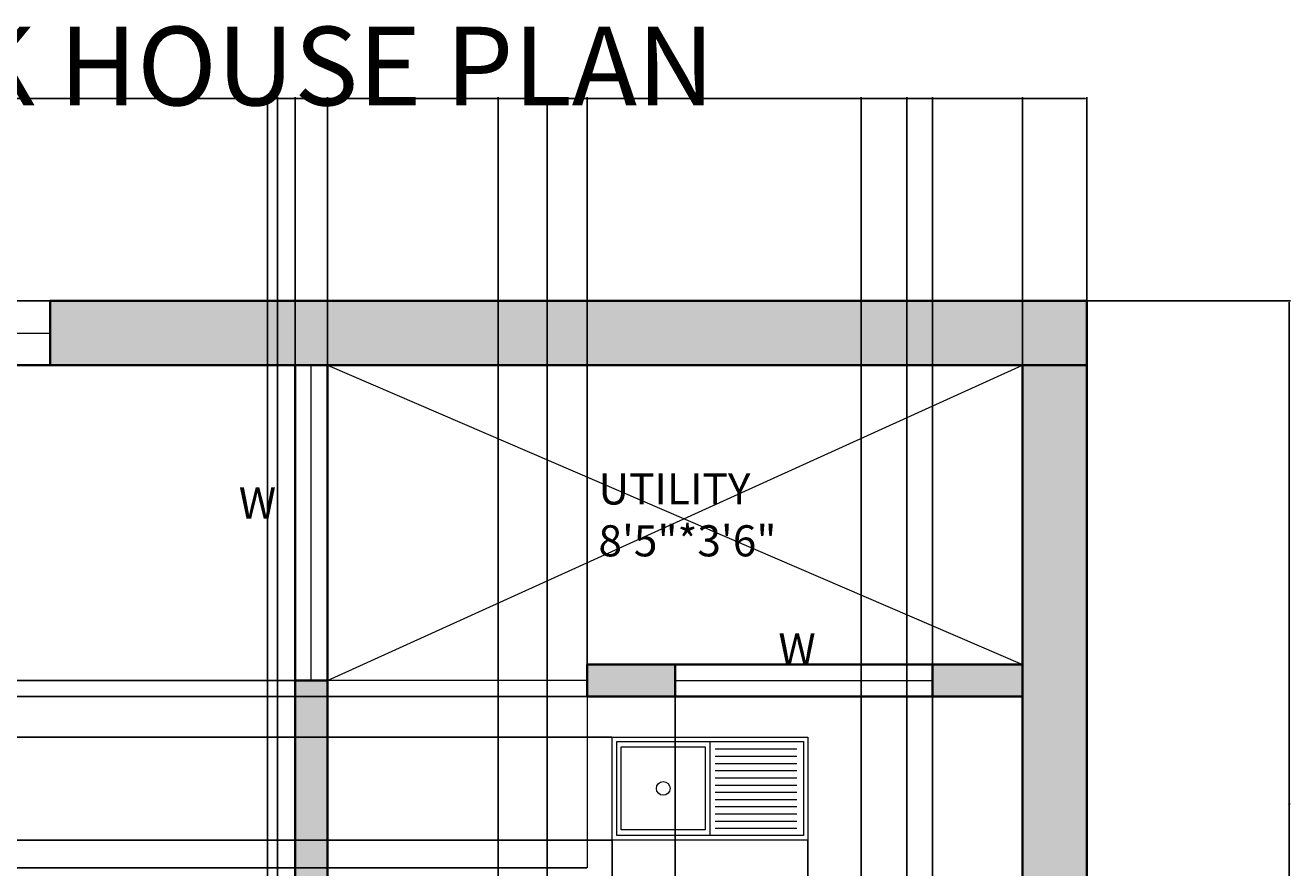
# Model space of a CAD drawing. Units: inches. Extents: x 2035 to 2384, y 1427 to 2020.
# Tile 7 of 7: x 2206 to 2383, y 1902 to 2020. Entities that reach past the tile are written whole.
import ezdxf

# ---------------------------------------------------------------- set-up
doc = ezdxf.new("R2010")
doc.units = ezdxf.units.IN
for name, color, linetype, lineweight in [('A-ANNO-DIMS', 2, 'Continuous', 18), ('A-ANNO-IDEN', 201, 'Continuous', 18), ('A-ANNO-TITL', 7, 'Continuous', 35), ('A-AREA-IDEN', 201, 'Continuous', 18), ('A-FLOR-CABN', 71, 'Continuous', 18), ('A-FLOR-FIXT', 9, 'Continuous', 18), ('A-FLOR-FIXT-PATT', 9, 'Continuous', 13), ('A-FLOR-OPEN', 8, 'Continuous', 13), ('A-WALL-PATT', 140, 'Continuous', 13), ('C-PROP', 7, 'Continuous', 25), ('WALL', 140, 'Continuous', 35), ('WIN', 230, 'Continuous', 18)]:
    doc.layers.add(name, color=color, linetype=linetype, lineweight=lineweight)
doc.styles.get("Standard").update_dxf_attribs({"font": 'arial.ttf'})
doc.dimstyles.get("Standard").update_dxf_attribs({"dimtxt": 0.18, "dimasz": 0.18, "dimexe": 0.18, "dimexo": 0.0625, "dimgap": 0.09, "dimtad": 0, "dimtih": 1, "dimtoh": 1, "dimdec": 4, "dimzin": 0, "dimdsep": 46, "dimtxsty": 'Standard', "dimcen": 0.09, "dimadec": 0, "dimazin": 0, "dimtfac": 1, "dimtdec": 4, "dimtofl": 0, "dimtmove": 0, "dimatfit": 3, "dimfxl": 1, "dimtolj": 1, "dimtzin": 0, "dimarcsym": 0})

# ---------------------------------------------------------------- blocks, each defined once
blk = doc.blocks.new('WIN-BEDROOM')
blk.add_line((0, 4.5), (63.76, 4.5))
blk.add_lwpolyline([(0, 9), (63.76, 9), (63.76, 0), (0, 0)], close=True)
blk = doc.blocks.new('*D22')
at = {"layer": 'A-ANNO-DIMS', "color": 0, "lineweight": -2, "transparency": 16777216}
for p, q in [((2114.75, 1981.44), (2114.75, 2009.96)), ((2114.93, 2009.78), (2234.46, 2009.78)), ((2354.57, 2009.78), (2235.04, 2009.78)), ((2354.75, 1981.44), (2354.75, 2009.96))]:
    blk.add_line(p, q, dxfattribs=at)
at = {"layer": 'A-ANNO-DIMS', "color": 0, "lineweight": 100, "transparency": 16777216}
for points in [[(2114.93, 2009.81), (2114.93, 2009.75), (2114.75, 2009.78)], [(2354.57, 2009.81), (2354.57, 2009.75), (2354.75, 2009.78)]]:
    blk.add_solid(points, dxfattribs=at)
at = {"layer": 'Defpoints', "color": 0, "lineweight": 100, "transparency": 16777216}
for p in [(2354.75, 2009.78), (2114.75, 1981.38), (2354.75, 1981.38)]:
    blk.add_point(p, dxfattribs=at)
at = {"layer": 'A-ANNO-DIMS', "color": 0, "transparency": 16777216, "insert": (2234.75, 2009.78), "char_height": 0.18, "attachment_point": 5}
blk.add_mtext('\\A1;240', dxfattribs=at)
blk = doc.blocks.new('*D23')
at = {"layer": 'A-ANNO-DIMS', "color": 0, "lineweight": -2, "transparency": 16777216}
for p, q in [((2354.82, 1981.38), (2383.33, 1981.38)), ((2383.15, 1981.2), (2383.15, 1741.56)), ((2383.15, 1501.56), (2383.15, 1741.2)), ((2354.82, 1501.38), (2383.33, 1501.38))]:
    blk.add_line(p, q, dxfattribs=at)
at = {"layer": 'A-ANNO-DIMS', "color": 0, "lineweight": 100, "transparency": 16777216}
for points in [[(2383.12, 1981.2), (2383.18, 1981.2), (2383.15, 1981.38)], [(2383.12, 1501.56), (2383.18, 1501.56), (2383.15, 1501.38)]]:
    blk.add_solid(points, dxfattribs=at)
at = {"layer": 'Defpoints', "color": 0, "lineweight": 100, "transparency": 16777216}
for p in [(2354.75, 1981.38), (2383.15, 1981.38), (2354.75, 1501.38)]:
    blk.add_point(p, dxfattribs=at)
at = {"layer": 'A-ANNO-DIMS', "color": 0, "transparency": 16777216, "insert": (2383.15, 1741.38), "char_height": 0.18, "attachment_point": 5}
blk.add_mtext('\\A1;480', dxfattribs=at)
blk = doc.blocks.new('*D25')
at = {"layer": 'A-ANNO-DIMS', "color": 0, "lineweight": -2, "transparency": 16777216}
for p, q in [((2241.25, 1503.69), (2241.25, 2009.96)), ((2241.43, 2009.78), (2256.26, 2009.78)), ((2272.01, 2009.78), (2257.18, 2009.78)), ((2272.19, 1503.69), (2272.19, 2009.96))]:
    blk.add_line(p, q, dxfattribs=at)
at = {"layer": 'A-ANNO-DIMS', "color": 0, "lineweight": 100, "transparency": 16777216}
for points in [[(2241.43, 2009.81), (2241.43, 2009.75), (2241.25, 2009.78)], [(2272.01, 2009.81), (2272.01, 2009.75), (2272.19, 2009.78)]]:
    blk.add_solid(points, dxfattribs=at)
at = {"layer": 'Defpoints', "color": 0, "lineweight": 100, "transparency": 16777216}
for p in [(2272.19, 2009.78), (2241.25, 1503.63), (2272.19, 1503.63)]:
    blk.add_point(p, dxfattribs=at)
at = {"layer": 'A-ANNO-DIMS', "color": 0, "transparency": 16777216, "insert": (2256.72, 2009.78), "char_height": 0.18, "attachment_point": 5}
blk.add_mtext('\\A1;30.935', dxfattribs=at)
blk = doc.blocks.new('*D26')
at = {"layer": 'A-ANNO-DIMS', "color": 0, "lineweight": -2, "transparency": 16777216}
for p, q in [((2272.19, 1506.56), (2272.19, 2009.96)), ((2272.37, 2009.78), (2297.26, 2009.78)), ((2322.93, 2009.78), (2298.04, 2009.78)), ((2323.11, 1506.56), (2323.11, 2009.96))]:
    blk.add_line(p, q, dxfattribs=at)
at = {"layer": 'A-ANNO-DIMS', "color": 0, "lineweight": 100, "transparency": 16777216}
for points in [[(2272.37, 2009.81), (2272.37, 2009.75), (2272.19, 2009.78)], [(2322.93, 2009.81), (2322.93, 2009.75), (2323.11, 2009.78)]]:
    blk.add_solid(points, dxfattribs=at)
at = {"layer": 'Defpoints', "color": 0, "lineweight": 100, "transparency": 16777216}
for p in [(2323.11, 2009.78), (2272.19, 1506.5), (2323.11, 1506.5)]:
    blk.add_point(p, dxfattribs=at)
at = {"layer": 'A-ANNO-DIMS', "color": 0, "transparency": 16777216, "insert": (2297.65, 2009.78), "char_height": 0.18, "attachment_point": 5}
blk.add_mtext('\\A1;50.92', dxfattribs=at)
blk = doc.blocks.new('*D42')
at = {"layer": 'A-ANNO-DIMS', "color": 0, "lineweight": -2, "transparency": 16777216}
for p, q in [((2297.05, 1925.82), (2297.05, 1427.17)), ((2333.11, 1925.82), (2333.11, 1427.17)), ((2297.23, 1427.35), (2314.69, 1427.35)), ((2332.93, 1427.35), (2315.47, 1427.35))]:
    blk.add_line(p, q, dxfattribs=at)
at = {"layer": 'A-ANNO-DIMS', "color": 0, "lineweight": 100, "transparency": 16777216}
for points in [[(2297.23, 1427.38), (2297.23, 1427.32), (2297.05, 1427.35)], [(2332.93, 1427.38), (2332.93, 1427.32), (2333.11, 1427.35)]]:
    blk.add_solid(points, dxfattribs=at)
at = {"layer": 'Defpoints', "color": 0, "lineweight": 100, "transparency": 16777216}
for p in [(2297.05, 1925.88), (2333.11, 1925.88), (2333.11, 1427.35)]:
    blk.add_point(p, dxfattribs=at)
at = {"layer": 'A-ANNO-DIMS', "color": 0, "transparency": 16777216, "insert": (2315.08, 1427.35), "char_height": 0.18, "attachment_point": 5}
blk.add_mtext('\\A1;36.06', dxfattribs=at)
blk = doc.blocks.new('*D43')
at = {"layer": 'A-ANNO-DIMS', "color": 0, "lineweight": -2, "transparency": 16777216}
for p, q in [((2243.69, 1972.38), (2035.17, 1972.38)), ((2035.35, 1972.2), (2035.35, 1950.44)), ((2035.35, 1928.31), (2035.35, 1950.07)), ((2243.69, 1928.13), (2035.17, 1928.13))]:
    blk.add_line(p, q, dxfattribs=at)
at = {"layer": 'A-ANNO-DIMS', "color": 0, "lineweight": 100, "transparency": 16777216}
for points in [[(2035.32, 1972.2), (2035.38, 1972.2), (2035.35, 1972.38)], [(2035.32, 1928.31), (2035.38, 1928.31), (2035.35, 1928.13)]]:
    blk.add_solid(points, dxfattribs=at)
at = {"layer": 'Defpoints', "color": 0, "lineweight": 100, "transparency": 16777216}
for p in [(2035.35, 1972.38), (2243.75, 1972.38), (2243.75, 1928.13)]:
    blk.add_point(p, dxfattribs=at)
at = {"layer": 'A-ANNO-DIMS', "color": 0, "transparency": 16777216, "insert": (2035.35, 1950.26), "char_height": 0.18, "attachment_point": 5}
blk.add_mtext('\\A1;44.25', dxfattribs=at)
blk = doc.blocks.new('*D44')
at = {"layer": 'A-ANNO-DIMS', "color": 0, "lineweight": -2, "transparency": 16777216}
for p, q in [((2284.64, 1925.88), (2035.17, 1925.88)), ((2035.35, 1925.7), (2035.35, 1914.06)), ((2035.35, 1902.06), (2035.35, 1913.7)), ((2284.64, 1901.88), (2035.17, 1901.88))]:
    blk.add_line(p, q, dxfattribs=at)
at = {"layer": 'A-ANNO-DIMS', "color": 0, "lineweight": 100, "transparency": 16777216}
for points in [[(2035.32, 1925.7), (2035.38, 1925.7), (2035.35, 1925.88)], [(2035.32, 1902.06), (2035.38, 1902.06), (2035.35, 1901.88)]]:
    blk.add_solid(points, dxfattribs=at)
at = {"layer": 'Defpoints', "color": 0, "lineweight": 100, "transparency": 16777216}
for p in [(2284.7, 1925.88), (2035.35, 1901.88), (2284.7, 1901.88)]:
    blk.add_point(p, dxfattribs=at)
at = {"layer": 'A-ANNO-DIMS', "color": 0, "transparency": 16777216, "insert": (2035.35, 1913.88), "char_height": 0.18, "attachment_point": 5}
blk.add_mtext('\\A1;24', dxfattribs=at)
blk = doc.blocks.new('*D46')
at = {"layer": 'A-ANNO-DIMS', "color": 0, "lineweight": -2, "transparency": 16777216}
for p, q in [((2288.19, 1905.68), (2288.19, 1427.17)), ((2315.66, 1905.68), (2315.66, 1427.17)), ((2288.37, 1427.35), (2301.53, 1427.35)), ((2315.48, 1427.35), (2302.32, 1427.35))]:
    blk.add_line(p, q, dxfattribs=at)
at = {"layer": 'A-ANNO-DIMS', "color": 0, "lineweight": 100, "transparency": 16777216}
for points in [[(2288.37, 1427.38), (2288.37, 1427.32), (2288.19, 1427.35)], [(2315.48, 1427.38), (2315.48, 1427.32), (2315.66, 1427.35)]]:
    blk.add_solid(points, dxfattribs=at)
at = {"layer": 'Defpoints', "color": 0, "lineweight": 100, "transparency": 16777216}
for p in [(2288.19, 1905.75), (2315.66, 1905.75), (2315.66, 1427.35)]:
    blk.add_point(p, dxfattribs=at)
at = {"layer": 'A-ANNO-DIMS', "color": 0, "transparency": 16777216, "insert": (2301.92, 1427.35), "char_height": 0.18, "attachment_point": 5}
blk.add_mtext('\\A1;27.47', dxfattribs=at)
blk = doc.blocks.new('*D47')
at = {"layer": 'A-ANNO-DIMS', "color": 0, "lineweight": -2, "transparency": 16777216}
for p, q in [((2288.13, 1920.21), (2035.17, 1920.21)), ((2035.35, 1920.03), (2035.35, 1913.16)), ((2035.35, 1905.93), (2035.35, 1912.8)), ((2288.13, 1905.75), (2035.17, 1905.75))]:
    blk.add_line(p, q, dxfattribs=at)
at = {"layer": 'A-ANNO-DIMS', "color": 0, "lineweight": 100, "transparency": 16777216}
for points in [[(2035.32, 1920.03), (2035.38, 1920.03), (2035.35, 1920.21)], [(2035.32, 1905.93), (2035.38, 1905.93), (2035.35, 1905.75)]]:
    blk.add_solid(points, dxfattribs=at)
at = {"layer": 'Defpoints', "color": 0, "lineweight": 100, "transparency": 16777216}
for p in [(2035.35, 1920.21), (2288.19, 1920.21), (2288.19, 1905.75)]:
    blk.add_point(p, dxfattribs=at)
at = {"layer": 'A-ANNO-DIMS', "color": 0, "transparency": 16777216, "insert": (2035.35, 1912.98), "char_height": 0.18, "attachment_point": 5}
blk.add_mtext('\\A1;14.463', dxfattribs=at)
blk = doc.blocks.new('*D54')
at = {"layer": 'A-ANNO-DIMS', "color": 0, "lineweight": -2, "transparency": 16777216}
for p, q in [((2239.88, 1811.3), (2239.88, 2009.96)), ((2240.06, 2009.78), (2259.08, 2009.78)), ((2278.89, 2009.78), (2259.87, 2009.78)), ((2279.07, 1811.3), (2279.07, 2009.96))]:
    blk.add_line(p, q, dxfattribs=at)
at = {"layer": 'A-ANNO-DIMS', "color": 0, "lineweight": 100, "transparency": 16777216}
for points in [[(2240.06, 2009.81), (2240.06, 2009.75), (2239.88, 2009.78)], [(2278.89, 2009.81), (2278.89, 2009.75), (2279.07, 2009.78)]]:
    blk.add_solid(points, dxfattribs=at)
at = {"layer": 'Defpoints', "color": 0, "lineweight": 100, "transparency": 16777216}
for p in [(2279.07, 2009.78), (2239.88, 1811.24), (2279.07, 1811.24)]:
    blk.add_point(p, dxfattribs=at)
at = {"layer": 'A-ANNO-DIMS', "color": 0, "transparency": 16777216, "insert": (2259.47, 2009.78), "char_height": 0.18, "attachment_point": 5}
blk.add_mtext('\\A1;39.19', dxfattribs=at)
blk = doc.blocks.new('*D58')
at = {"layer": 'A-ANNO-DIMS', "color": 0, "lineweight": -2, "transparency": 16777216}
for p, q in [((2248.25, 1928.19), (2248.25, 2009.96)), ((2248.43, 2009.78), (2266.08, 2009.78)), ((2284.52, 2009.78), (2266.87, 2009.78)), ((2284.7, 1928.19), (2284.7, 2009.96))]:
    blk.add_line(p, q, dxfattribs=at)
at = {"layer": 'A-ANNO-DIMS', "color": 0, "lineweight": 100, "transparency": 16777216}
for points in [[(2248.43, 2009.81), (2248.43, 2009.75), (2248.25, 2009.78)], [(2284.52, 2009.81), (2284.52, 2009.75), (2284.7, 2009.78)]]:
    blk.add_solid(points, dxfattribs=at)
at = {"layer": 'Defpoints', "color": 0, "lineweight": 100, "transparency": 16777216}
for p in [(2284.7, 2009.78), (2248.25, 1928.13), (2284.7, 1928.13)]:
    blk.add_point(p, dxfattribs=at)
at = {"layer": 'A-ANNO-DIMS', "color": 0, "transparency": 16777216, "insert": (2266.48, 2009.78), "char_height": 0.18, "attachment_point": 5}
blk.add_mtext('\\A1;36.45', dxfattribs=at)
blk = doc.blocks.new('*D59')
at = {"layer": 'A-ANNO-DIMS', "color": 0, "lineweight": -2, "transparency": 16777216}
for p, q in [((2354.82, 1981.38), (2383.33, 1981.38)), ((2383.15, 1981.2), (2383.15, 1911.06)), ((2383.15, 1840.56), (2383.15, 1910.7)), ((2345.82, 1840.38), (2383.33, 1840.38))]:
    blk.add_line(p, q, dxfattribs=at)
at = {"layer": 'A-ANNO-DIMS', "color": 0, "lineweight": 100, "transparency": 16777216}
for points in [[(2383.12, 1981.2), (2383.18, 1981.2), (2383.15, 1981.38)], [(2383.12, 1840.56), (2383.18, 1840.56), (2383.15, 1840.38)]]:
    blk.add_solid(points, dxfattribs=at)
at = {"layer": 'Defpoints', "color": 0, "lineweight": 100, "transparency": 16777216}
for p in [(2354.75, 1981.38), (2383.15, 1981.38), (2345.75, 1840.38)]:
    blk.add_point(p, dxfattribs=at)
at = {"layer": 'A-ANNO-DIMS', "color": 0, "transparency": 16777216, "insert": (2383.15, 1910.88), "char_height": 0.18, "attachment_point": 5}
blk.add_mtext('\\A1;141', dxfattribs=at)
blk = doc.blocks.new('*D60')
at = {"layer": 'A-ANNO-DIMS', "color": 0, "lineweight": -2, "transparency": 16777216}
for p, q in [((2193.76, 1860.83), (2193.76, 2009.96)), ((2193.94, 2009.78), (2218.54, 2009.78)), ((2243.57, 2009.78), (2218.97, 2009.78)), ((2243.75, 1840.44), (2243.75, 2009.96))]:
    blk.add_line(p, q, dxfattribs=at)
at = {"layer": 'A-ANNO-DIMS', "color": 0, "lineweight": 100, "transparency": 16777216}
for points in [[(2193.94, 2009.81), (2193.94, 2009.75), (2193.76, 2009.78)], [(2243.57, 2009.81), (2243.57, 2009.75), (2243.75, 2009.78)]]:
    blk.add_solid(points, dxfattribs=at)
at = {"layer": 'Defpoints', "color": 0, "lineweight": 100, "transparency": 16777216}
for p in [(2243.75, 2009.78), (2193.76, 1860.77), (2243.75, 1840.38)]:
    blk.add_point(p, dxfattribs=at)
at = {"layer": 'A-ANNO-DIMS', "color": 0, "transparency": 16777216, "insert": (2218.75, 2009.78), "char_height": 0.18, "attachment_point": 5}
blk.add_mtext('\\A1;50', dxfattribs=at)
blk = doc.blocks.new('*D68')
at = {"layer": 'A-ANNO-DIMS', "color": 0, "lineweight": -2, "transparency": 16777216}
for p, q in [((2329.51, 1685.44), (2329.51, 2009.96)), ((2329.69, 2009.78), (2337.25, 2009.78)), ((2345.57, 2009.78), (2338.02, 2009.78)), ((2345.75, 1685.44), (2345.75, 2009.96))]:
    blk.add_line(p, q, dxfattribs=at)
at = {"layer": 'A-ANNO-DIMS', "color": 0, "lineweight": 100, "transparency": 16777216}
for points in [[(2329.69, 2009.81), (2329.69, 2009.75), (2329.51, 2009.78)], [(2345.57, 2009.81), (2345.57, 2009.75), (2345.75, 2009.78)]]:
    blk.add_solid(points, dxfattribs=at)
at = {"layer": 'Defpoints', "color": 0, "lineweight": 100, "transparency": 16777216}
for p in [(2345.75, 2009.78), (2329.51, 1685.38), (2345.75, 1685.38)]:
    blk.add_point(p, dxfattribs=at)
at = {"layer": 'A-ANNO-DIMS', "color": 0, "transparency": 16777216, "insert": (2337.63, 2009.78), "char_height": 0.18, "attachment_point": 5}
blk.add_mtext('\\A1;16.24', dxfattribs=at)
blk = doc.blocks.new('*D69')
at = {"layer": 'A-ANNO-DIMS', "color": 0, "lineweight": -2, "transparency": 16777216}
for p, q in [((2333.11, 1930.44), (2333.11, 2009.96)), ((2333.29, 2009.78), (2338.98, 2009.78)), ((2345.57, 2009.78), (2339.89, 2009.78)), ((2345.75, 1930.44), (2345.75, 2009.96))]:
    blk.add_line(p, q, dxfattribs=at)
at = {"layer": 'A-ANNO-DIMS', "color": 0, "lineweight": 100, "transparency": 16777216}
for points in [[(2333.29, 2009.81), (2333.29, 2009.75), (2333.11, 2009.78)], [(2345.57, 2009.81), (2345.57, 2009.75), (2345.75, 2009.78)]]:
    blk.add_solid(points, dxfattribs=at)
at = {"layer": 'Defpoints', "color": 0, "lineweight": 100, "transparency": 16777216}
for p in [(2345.75, 2009.78), (2333.11, 1930.38), (2345.75, 1930.38)]:
    blk.add_point(p, dxfattribs=at)
at = {"layer": 'A-ANNO-DIMS', "color": 0, "transparency": 16777216, "insert": (2339.43, 2009.78), "char_height": 0.18, "attachment_point": 5}
blk.add_mtext('\\A1;12.643', dxfattribs=at)
blk = doc.blocks.new('*D70')
at = {"layer": 'A-ANNO-DIMS', "color": 0, "lineweight": -2, "transparency": 16777216}
for p, q in [((2188.25, 1804.46), (2188.25, 2009.96)), ((2188.43, 2009.78), (2213.67, 2009.78)), ((2239.7, 2009.78), (2214.46, 2009.78)), ((2239.88, 1811.3), (2239.88, 2009.96))]:
    blk.add_line(p, q, dxfattribs=at)
at = {"layer": 'A-ANNO-DIMS', "color": 0, "lineweight": 100, "transparency": 16777216}
for points in [[(2188.43, 2009.81), (2188.43, 2009.75), (2188.25, 2009.78)], [(2239.7, 2009.81), (2239.7, 2009.75), (2239.88, 2009.78)]]:
    blk.add_solid(points, dxfattribs=at)
at = {"layer": 'Defpoints', "color": 0, "lineweight": 100, "transparency": 16777216}
for p in [(2239.88, 2009.78), (2239.88, 1811.24), (2188.25, 1804.39)]:
    blk.add_point(p, dxfattribs=at)
at = {"layer": 'A-ANNO-DIMS', "color": 0, "transparency": 16777216, "insert": (2214.07, 2009.78), "char_height": 0.18, "attachment_point": 5}
blk.add_mtext('\\A1;51.62', dxfattribs=at)

msp = doc.modelspace()

# ---------------------------------------------------------------- hatches: boundary and pattern name
at = {"layer": 'A-FLOR-FIXT-PATT'}
h = msp.add_hatch(dxfattribs=at)
h.set_pattern_fill('ANSI31', color=256, scale=0.3183684, angle=-45, style=0)
h.paths.add_polyline_path([(2302.6228, 1907.4149), (2314.1183, 1907.4149), (2314.1183, 1918.5404), (2302.6228, 1918.5404)])
at = {"layer": 'A-WALL-PATT'}
h = msp.add_hatch(color=256, dxfattribs=at)
h.dxf.hatch_style = 1
h.paths.add_polyline_path([(2145.6215, 1981.3816), (2123.7529, 1981.3816), (2123.7529, 1972.3816), (2145.6215, 1972.3816)])
h.paths.add_polyline_path([(2354.7529, 1981.3816), (2209.3767, 1981.3816), (2209.3767, 1972.3816), (2354.7529, 1972.3816)])
h.paths.add_polyline_path([(2123.7529, 1981.3816), (2114.7529, 1981.3816), (2114.7529, 1505.8816), (2123.7529, 1505.8816)])
h.paths.add_polyline_path([(2248.2529, 1928.1316), (2243.7529, 1928.1316), (2243.7529, 1840.3816), (2248.2529, 1840.3816)])
h.paths.add_polyline_path([(2297.0514, 1930.3816), (2284.6994, 1930.3816), (2284.6994, 1925.8816), (2297.0514, 1925.8816)])
h.paths.add_polyline_path([(2345.7529, 1930.3816), (2333.1098, 1930.3816), (2333.1098, 1925.8816), (2345.7529, 1925.8816)])
h.paths.add_polyline_path([(2354.7529, 1972.3816), (2345.7529, 1972.3816), (2345.7529, 1501.3816), (2354.7529, 1501.3816)])
h.paths.add_polyline_path([(2188.2529, 1835.8816), (2183.7529, 1835.8816), (2183.7529, 1831.3677), (2184.207, 1831.3677), (2188.2529, 1831.3677)])
h.paths.add_polyline_path([(2188.2529, 1804.3949), (2184.207, 1804.3949), (2183.7529, 1804.3949), (2183.7529, 1685.3816), (2188.2529, 1685.3816)])
h.paths.add_polyline_path([(2273.5087, 1840.3816), (2241.0146, 1840.3816), (2241.0146, 1835.8816), (2273.5087, 1835.8816)])
h.paths.add_polyline_path([(2345.7529, 1840.3816), (2310.4577, 1840.3816), (2310.4577, 1835.8816), (2345.7529, 1835.8816)])
h.paths.add_polyline_path([(2161.9064, 1524.4315), (2196.2972, 1524.4315), (2196.2972, 1533.4306), (2161.9064, 1533.4306)], flags=9)
h.paths.add_polyline_path([(2279.3058, 1589.7515), (2308.9483, 1589.7515), (2308.9483, 1598.7506), (2279.3058, 1598.7506)], flags=9)
h.paths.add_polyline_path([(2242.9684, 1662.1655), (2279.0513, 1662.1655), (2279.0513, 1671.1647), (2242.9684, 1671.1647)], flags=9)
h.paths.add_polyline_path([(2154.6483, 1622.8242), (2195.1309, 1622.8242), (2195.1309, 1639.1195), (2154.6483, 1639.1195)], flags=9)
h.paths.add_polyline_path([(2138.8708, 1715.378), (2162.5199, 1715.378), (2162.5199, 1731.6734), (2138.8708, 1731.6734)], flags=9)
h.paths.add_polyline_path([(2135.5598, 1791.707), (2165.1993, 1791.707), (2165.1993, 1808.0024), (2135.5598, 1808.0024)], flags=9)
h.paths.add_polyline_path([(2245.1071, 1740.4502), (2279.0303, 1740.4502), (2279.0303, 1756.7455), (2245.1071, 1756.7455)], flags=9)
h.paths.add_polyline_path([(2284.7312, 1866.5552), (2313.6916, 1866.5552), (2313.6916, 1890.2034), (2284.7312, 1890.2034)], flags=9)
h.paths.add_polyline_path([(2139.9071, 1874.6496), (2173.8303, 1874.6496), (2173.8303, 1890.9449), (2139.9071, 1890.9449)], flags=9)
h = msp.add_hatch(color=256, dxfattribs=at)
h.dxf.hatch_style = 1
h.paths.add_polyline_path([(2236.7529, 1556.8816), (2209.3767, 1556.8816), (2209.3767, 1547.8816), (2236.7529, 1547.8816)])
h.paths.add_polyline_path([(2241.2529, 1680.8816), (2236.7529, 1680.8816), (2236.7529, 1547.8816), (2241.2529, 1547.8816)])
h.paths.add_polyline_path([(2241.2529, 1505.8816), (2114.7529, 1505.8816), (2114.7529, 1501.3816), (2241.2529, 1501.3816)])
h.paths.add_polyline_path([(2242.179, 1683.1823), (2242.179, 1685.3816), (2234.769, 1685.3816), (2234.769, 1680.8816), (2242.179, 1680.8816)])
h.paths.add_polyline_path([(2286.8795, 1685.3816), (2272.8549, 1685.3816), (2272.8549, 1683.1823), (2272.8549, 1680.8816), (2286.8795, 1680.8816)])
h.paths.add_polyline_path([(2345.7529, 1685.3816), (2329.513, 1685.3816), (2329.513, 1680.8816), (2345.7529, 1680.8816)])
h.paths.add_polyline_path([(2279.3058, 1589.7515), (2308.9483, 1589.7515), (2308.9483, 1598.7506), (2279.3058, 1598.7506)], flags=9)
h.paths.add_polyline_path([(2242.9684, 1662.1655), (2279.0513, 1662.1655), (2279.0513, 1671.1647), (2242.9684, 1671.1647)], flags=9)
h.paths.add_polyline_path([(2154.6483, 1622.8242), (2195.1309, 1622.8242), (2195.1309, 1639.1195), (2154.6483, 1639.1195)], flags=9)
h.paths.add_polyline_path([(2138.8708, 1715.378), (2162.5199, 1715.378), (2162.5199, 1731.6734), (2138.8708, 1731.6734)], flags=9)
h.paths.add_polyline_path([(2135.5598, 1791.707), (2165.1993, 1791.707), (2165.1993, 1808.0024), (2135.5598, 1808.0024)], flags=9)
h.paths.add_polyline_path([(2245.1071, 1740.4502), (2279.0303, 1740.4502), (2279.0303, 1756.7455), (2245.1071, 1756.7455)], flags=9)
h.paths.add_polyline_path([(2284.7312, 1866.5552), (2313.6916, 1866.5552), (2313.6916, 1890.2034), (2284.7312, 1890.2034)], flags=9)
h.paths.add_polyline_path([(2284.6985, 1943.1527), (2309.7208, 1943.1527), (2309.7208, 1959.448), (2284.6985, 1959.448)], flags=9)
h.paths.add_polyline_path([(2139.9071, 1874.6496), (2173.8303, 1874.6496), (2173.8303, 1890.9449), (2139.9071, 1890.9449)], flags=9)
h = msp.add_hatch(color=256, dxfattribs=at)
h.dxf.hatch_style = 1
h.paths.add_polyline_path([(2201.0146, 1840.3816), (2123.7529, 1840.3816), (2123.7529, 1835.8816), (2201.0146, 1835.8816)])
h.paths.add_polyline_path([(2136.2543, 1763.8816), (2123.7529, 1763.8816), (2123.7529, 1759.3816), (2136.2543, 1759.3816)])
h.paths.add_polyline_path([(2183.7529, 1763.8816), (2169.7769, 1763.8816), (2169.7769, 1759.3816), (2183.7529, 1759.3816)])
h.paths.add_polyline_path([(2152.8338, 1685.1369), (2152.8338, 1685.3816), (2123.7529, 1685.3816), (2123.7529, 1680.8816), (2152.8338, 1680.8816)])
h.paths.add_polyline_path([(2194.769, 1685.3816), (2181.2028, 1685.3816), (2181.2028, 1685.1369), (2181.2028, 1680.8816), (2194.769, 1680.8816)])
h.paths.add_polyline_path([(2145.6215, 1556.8816), (2123.7529, 1556.8816), (2123.7529, 1547.8816), (2145.6215, 1547.8816)])
h.paths.add_polyline_path([(2161.9064, 1524.4315), (2196.2972, 1524.4315), (2196.2972, 1533.4306), (2161.9064, 1533.4306)], flags=9)
h.paths.add_polyline_path([(2279.3058, 1589.7515), (2308.9483, 1589.7515), (2308.9483, 1598.7506), (2279.3058, 1598.7506)], flags=9)
h.paths.add_polyline_path([(2242.9684, 1662.1655), (2279.0513, 1662.1655), (2279.0513, 1671.1647), (2242.9684, 1671.1647)], flags=9)
h.paths.add_polyline_path([(2154.6483, 1622.8242), (2195.1309, 1622.8242), (2195.1309, 1639.1195), (2154.6483, 1639.1195)], flags=9)
h.paths.add_polyline_path([(2138.8708, 1715.378), (2162.5199, 1715.378), (2162.5199, 1731.6734), (2138.8708, 1731.6734)], flags=9)
h.paths.add_polyline_path([(2135.5598, 1791.707), (2165.1993, 1791.707), (2165.1993, 1808.0024), (2135.5598, 1808.0024)], flags=9)
h.paths.add_polyline_path([(2245.1071, 1740.4502), (2279.0303, 1740.4502), (2279.0303, 1756.7455), (2245.1071, 1756.7455)], flags=9)
h.paths.add_polyline_path([(2284.7312, 1866.5552), (2313.6916, 1866.5552), (2313.6916, 1890.2034), (2284.7312, 1890.2034)], flags=9)
h.paths.add_polyline_path([(2284.6985, 1943.1527), (2309.7208, 1943.1527), (2309.7208, 1959.448), (2284.6985, 1959.448)], flags=9)
h.paths.add_polyline_path([(2139.9071, 1874.6496), (2173.8303, 1874.6496), (2173.8303, 1890.9449), (2139.9071, 1890.9449)], flags=9)

# ---------------------------------------------------------------- linework, layer by layer
at = {"layer": 'A-FLOR-CABN'}
msp.add_line((2284.6994, 1925.8816), (2284.6994, 1901.8816), dxfattribs=at)
at = {"layer": 'A-FLOR-FIXT'}
msp.add_line((2301.9245, 1906.3903), (2301.9245, 1919.5645), dxfattribs=at)
for points in [[(2288.1887, 1920.2089), (2315.6602, 1920.2089), (2315.6602, 1905.7459), (2288.1887, 1905.7459)], [(2288.8331, 1919.5645), (2315.0159, 1919.5645), (2315.0159, 1906.3903), (2288.8331, 1906.3903)], [(2289.4709, 1918.8363), (2301.2315, 1918.8363), (2301.2315, 1907.1852), (2289.4709, 1907.1852)]]:
    msp.add_lwpolyline(points, close=True, dxfattribs=at)
msp.add_circle((2295.3512, 1913.0108), 0.9599, dxfattribs=at)
at = {"layer": 'A-FLOR-OPEN'}
for p, q in [((2248.2529, 1928.1316), (2345.7529, 1972.3816)), ((2248.2529, 1972.3816), (2345.7529, 1930.3816)), ((2284.6994, 1928.1316), (2248.2529, 1928.1316))]:
    msp.add_line(p, q, dxfattribs=at)
at = {"layer": 'C-PROP'}
for p, q in [((2114.7529, 1981.3816), (2354.7529, 1981.3816)), ((2354.7529, 1981.3816), (2354.7529, 1501.3816))]:
    msp.add_line(p, q, dxfattribs=at)
msp.add_lwpolyline([(2114.7529, 1981.3816), (2354.7529, 1981.3816), (2354.7529, 1501.3816), (2114.7529, 1501.3816)], close=True, dxfattribs=at)
at = {"layer": 'WALL'}
for p, q in [((2123.7529, 1972.3816), (2243.7529, 1972.3816)), ((2243.7529, 1972.3816), (2243.7529, 1840.3816)), ((2248.2529, 1972.3816), (2248.2529, 1840.3816)), ((2284.6994, 1930.3816), (2345.7529, 1930.3816)), ((2284.6994, 1925.8816), (2284.6994, 1930.3816)), ((2284.6994, 1925.8816), (2345.7529, 1925.8816))]:
    msp.add_line(p, q, dxfattribs=at)
for points in [[(2209.3767, 1972.3816), (2354.7529, 1972.3816), (2354.7529, 1981.3816), (2209.3767, 1981.3816)], [(2345.7529, 1972.3816), (2354.7529, 1972.3816), (2354.7529, 1501.3816), (2345.7529, 1501.3816)], [(2297.0514, 1925.8816), (2284.6994, 1925.8816), (2284.6994, 1930.3816), (2297.0514, 1930.3816)], [(2333.1098, 1925.8816), (2345.7529, 1925.8816), (2345.7529, 1930.3816), (2333.1098, 1930.3816)], [(2243.7529, 1928.1316), (2248.2529, 1928.1316), (2248.2529, 1840.3816), (2243.7529, 1840.3816)]]:
    msp.add_lwpolyline(points, close=True, dxfattribs=at)
msp.add_lwpolyline([(2241.2529, 1552.3816), (2241.2529, 1505.8816), (2123.7529, 1505.8816), (2123.7529, 1972.3816), (2345.7529, 1972.3816), (2345.7529, 1503.6316), (2323.1125, 1503.6316)], dxfattribs=at)
at = {"layer": 'WIN'}
for p, q in [((2243.7529, 1928.1316), (2243.7529, 1972.3816)), ((2246.0029, 1928.1316), (2246.0029, 1972.3816)), ((2248.2529, 1972.3816), (2248.2529, 1930.3816)), ((2248.2529, 1930.3816), (2248.2529, 1928.1316)), ((2248.2529, 1928.1316), (2243.7529, 1928.1316)), ((2297.0514, 1928.1316), (2333.1098, 1928.1316))]:
    msp.add_line(p, q, dxfattribs=at)
msp.add_lwpolyline([(2297.0514, 1930.3816), (2333.1098, 1930.3816), (2333.1098, 1925.8816), (2297.0514, 1925.8816)], close=True, dxfattribs=at)

# ---------------------------------------------------------------- block references
msp.add_blockref('WIN-BEDROOM', (2145.6215, 1972.3816), dxfattribs=at)

# ---------------------------------------------------------------- texts
at = {"layer": 'A-ANNO-IDEN', "char_height": 4.367, "attachment_point": 1}
for insert in [(2235.8316, 1955.2231), (2311.5092, 1934.7486)]:
    msp.add_mtext_dynamic_manual_height_columns('W', width=88.030619, gutter_width=21.835, heights=[0], dxfattribs=dict(at, insert=insert))
at = {"layer": 'A-ANNO-TITL', "insert": (2168.3128, 2019.8582), "char_height": 11.035976, "attachment_point": 1}
msp.add_mtext_dynamic_manual_height_columns('2BHK HOUSE PLAN', width=742.455452, gutter_width=55.1799, heights=[0], dxfattribs=at)
at = {"layer": 'A-AREA-IDEN', "insert": (2286.2698, 1957.2005), "char_height": 4.367, "attachment_point": 1}
msp.add_mtext_dynamic_manual_height_columns('UTILITY\\P8\'5"*3\'6"', width=88.030619, gutter_width=21.835, heights=[0], dxfattribs=at)

# ---------------------------------------------------------------- dimensions: what is measured, and where the dimension line sits
at = {"layer": 'A-ANNO-DIMS'}
for base, p1, p2, override, picture, middle in [((2354.7529, 2009.7816), (2114.7529, 1981.3816), (2354.7529, 1981.3816), {"dimdec": 0, "dimlfac": 1, "dimrnd": 0, "dimzin": 0, "dimdsep": 46, "dimlunit": 2}, '*D22', (2234.7529, 2009.7816)), ((2239.8773, 2009.7816), (2188.2529, 1804.3949), (2239.8773, 1811.2357), {"dimdec": 2, "dimlfac": 1, "dimrnd": 0, "dimzin": 0, "dimdsep": 46, "dimlunit": 2}, '*D70', (2214.0651, 2009.7816)), ((2243.7529, 2009.7816), (2193.7559, 1860.7719), (2243.7529, 1840.3816), {"dimdec": 0, "dimlfac": 1, "dimrnd": 0, "dimzin": 0, "dimdsep": 46, "dimlunit": 2}, '*D60', (2218.7544, 2009.7816)), ((2279.066, 2009.7816), (2239.8773, 1811.2357), (2279.066, 1811.2357), {"dimdec": 2, "dimlfac": 1, "dimrnd": 0, "dimzin": 0, "dimdsep": 46, "dimlunit": 2}, '*D54', (2259.4717, 2009.7816)), ((2272.1881, 2009.7816), (2241.2529, 1503.6316), (2272.1881, 1503.6316), {"dimdec": 3, "dimlfac": 1, "dimrnd": 0, "dimzin": 0, "dimdsep": 46, "dimlunit": 2}, '*D25', (2256.7205, 2009.7816)), ((2284.6994, 2009.7816), (2248.2529, 1928.1316), (2284.6994, 1928.1316), {"dimdec": 2, "dimlfac": 1, "dimrnd": 0, "dimzin": 0, "dimdsep": 46, "dimlunit": 2}, '*D58', (2266.4762, 2009.7816)), ((2323.1125, 2009.7816), (2272.1881, 1506.4959), (2323.1125, 1506.4959), {"dimdec": 2, "dimlfac": 1, "dimrnd": 0, "dimzin": 0, "dimdsep": 46, "dimlunit": 2}, '*D26', (2297.6503, 2009.7816)), ((2345.7529, 2009.7816), (2329.513, 1685.3816), (2345.7529, 1685.3816), {"dimdec": 2, "dimlfac": 1, "dimrnd": 0, "dimzin": 0, "dimdsep": 46, "dimlunit": 2}, '*D68', (2337.633, 2009.7816)), ((2345.7529, 2009.7816), (2333.1098, 1930.3816), (2345.7529, 1930.3816), {"dimdec": 3, "dimlfac": 1, "dimrnd": 0, "dimzin": 0, "dimdsep": 46, "dimlunit": 2}, '*D69', (2339.4313, 2009.7816)), ((2333.1098, 1427.3483), (2297.0514, 1925.8816), (2333.1098, 1925.8816), {"dimdec": 2, "dimlfac": 1, "dimrnd": 0, "dimzin": 0, "dimdsep": 46, "dimlunit": 2}, '*D42', (2315.0806, 1427.3483)), ((2315.6602, 1427.3483), (2288.1887, 1905.7459), (2315.6602, 1905.7459), {"dimdec": 2, "dimlfac": 1, "dimrnd": 0, "dimzin": 0, "dimdsep": 46, "dimlunit": 2}, '*D46', (2301.9245, 1427.3483))]:
    dim = msp.add_linear_dim(base=base, p1=p1, p2=p2, dimstyle='Standard', override=override, dxfattribs=at)
    dim.commit()
    dim.dimension.update_dxf_attribs({"geometry": picture, "text_midpoint": middle})
for base, p1, p2, override, picture, middle in [((2383.1529, 1981.3816), (2345.7529, 1840.3816), (2354.7529, 1981.3816), {"dimdec": 0, "dimlfac": 1, "dimrnd": 0, "dimzin": 0, "dimdsep": 46, "dimlunit": 2}, '*D59', (2383.1529, 1910.8816)), ((2383.1529, 1981.3816), (2354.7529, 1501.3816), (2354.7529, 1981.3816), {"dimdec": 0, "dimlfac": 1, "dimrnd": 0, "dimzin": 0, "dimdsep": 46, "dimlunit": 2}, '*D23', (2383.1529, 1741.3816)), ((2035.3529, 1972.3816), (2243.7529, 1928.1316), (2243.7529, 1972.3816), {"dimdec": 2, "dimlfac": 1, "dimrnd": 0, "dimzin": 0, "dimdsep": 46, "dimlunit": 2}, '*D43', (2035.3529, 1950.2566)), ((2035.3529, 1901.8816), (2284.6994, 1925.8816), (2284.6994, 1901.8816), {"dimdec": 0, "dimlfac": 1, "dimrnd": 0, "dimzin": 0, "dimdsep": 46, "dimlunit": 2}, '*D44', (2035.3529, 1913.8816)), ((2035.3529, 1920.2089), (2288.1887, 1905.7459), (2288.1887, 1920.2089), {"dimdec": 3, "dimlfac": 1, "dimrnd": 0, "dimzin": 0, "dimdsep": 46, "dimlunit": 2}, '*D47', (2035.3529, 1912.9774))]:
    dim = msp.add_linear_dim(base=base, p1=p1, p2=p2, angle=90, dimstyle='Standard', override=override, dxfattribs=at)
    dim.commit()
    dim.dimension.update_dxf_attribs({"geometry": picture, "text_midpoint": middle})

doc.saveas('drawing.dxf')
